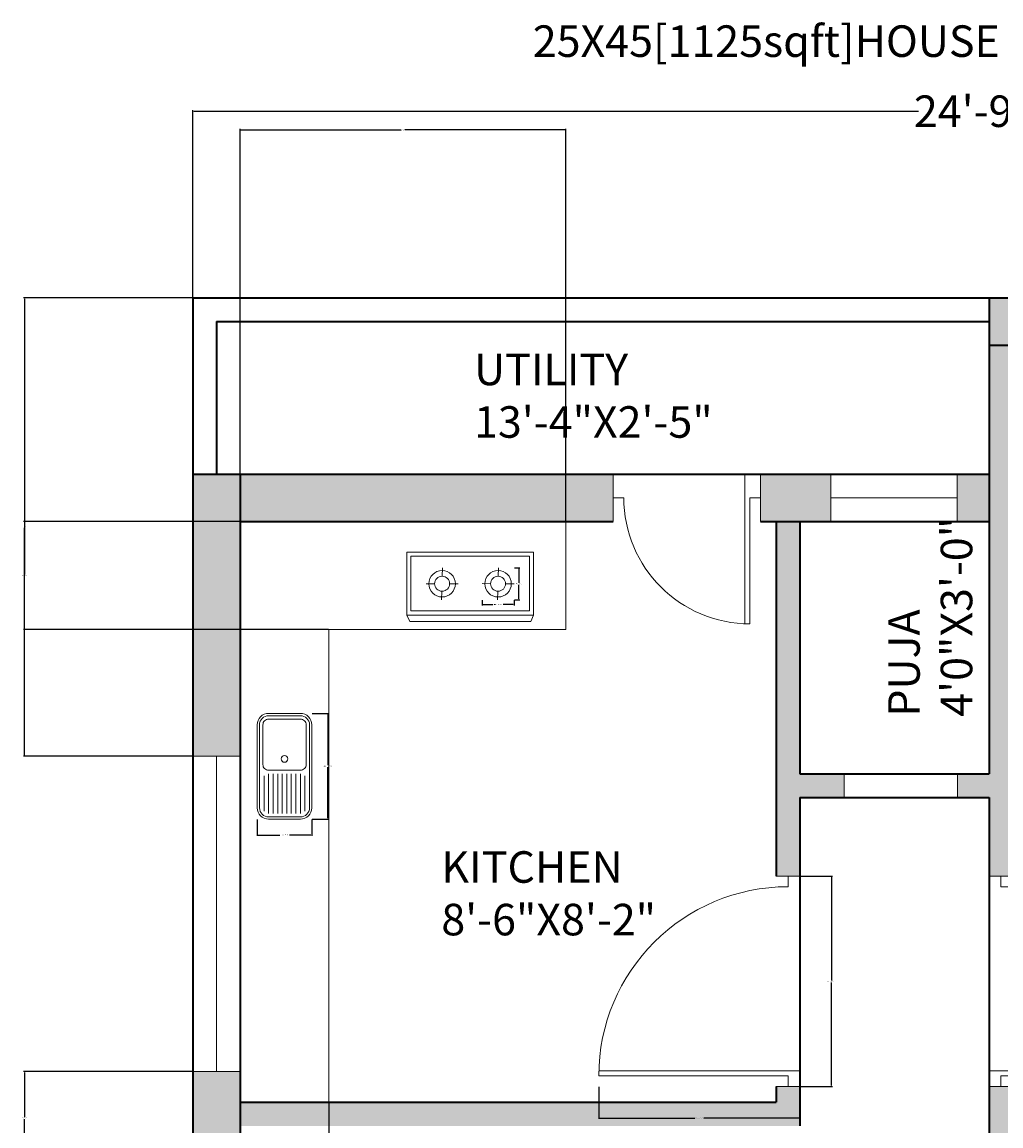
# Model space of a CAD drawing. Units: inches. Extents: x -13 to 349, y -556 to 61.
# Tile 5 of 6: x -13 to 174, y -149 to 61. Entities that reach past the tile are written whole.
import ezdxf

# ---------------------------------------------------------------- set-up
doc = ezdxf.new("R2010")
doc.units = ezdxf.units.IN
doc.header["$MEASUREMENT"] = 0
for name, color, linetype, lineweight in [('A-ANNO-DIMS', 2, 'Continuous', 18), ('A-ANNO-TEXT', 7, 'Continuous', 25), ('A-AREA-IDEN', 7, 'Continuous', 18), ('A-DOOR', 3, 'Continuous', 20), ('A-FLOR-CASE', 7, 'Continuous', 20), ('A-FLOR-OPEN', 1, 'Continuous', 13), ('A-GLAZ', 5, 'Continuous', 18), ('A-WALL', 7, 'Continuous', 35), ('A-WALL-PATT', 8, 'Continuous', 13), ('equipments', 7, 'Continuous', 18)]:
    doc.layers.add(name, color=color, linetype=linetype, lineweight=lineweight)
doc.styles.get("Standard").update_dxf_attribs({"font": 'arial.ttf'})
doc.dimstyles.get("Standard").update_dxf_attribs({"dimtxt": 0.18, "dimasz": 0.18, "dimexe": 0.18, "dimexo": 0.0625, "dimgap": 0.09, "dimtad": 0, "dimtih": 1, "dimtoh": 1, "dimdec": 0, "dimzin": 0, "dimdsep": 46, "dimlunit": 3, "dimtxsty": 'Standard', "dimcen": 0.09, "dimadec": 0, "dimazin": 0, "dimtfac": 1, "dimtdec": 0, "dimtofl": 0, "dimtmove": 0, "dimatfit": 3, "dimfxl": 1, "dimtolj": 1, "dimtzin": 0, "dimarcsym": 0})

# ---------------------------------------------------------------- blocks, each defined once
blk = doc.blocks.new('SINK_KITCHEN_SNGL')
for p, q in [((-39.5, -6), (-8.5, -6)), ((-36.5, -2), (36.5, -2)), ((-44.5, -38), (-44.5, -10)), ((-41.5, -10), (-6.5, -10)), ((-41.5, -14), (-6.5, -14)), ((-41.5, -18), (-6.5, -18)), ((44.5, -10), (44.5, -38)), ((-41.5, -22), (-6.5, -22)), ((-41.5, -26), (-6.5, -26)), ((-41.5, -30), (-6.5, -30)), ((-41.5, -34), (-6.5, -34)), ((-41.5, -38), (-6.5, -38)), ((-39.5, -42), (-8.5, -42)), ((36.5, -46), (-36.5, -46))]:
    blk.add_line(p, q)
at = {"flags": 128}
for points in [[(36.5, 0, -0.414214), (46.5, -10), (46.5, -38, -0.414214), (36.5, -48), (-36.5, -48, -0.414214), (-46.5, -38), (-46.5, -10, -0.414214), (-36.5, 0)], [(36.5, -5, -0.414214), (41.5, -10), (41.5, -38, -0.414214), (36.5, -43), (1.5, -43, -0.414214), (-3.5, -38), (-3.5, -10, -0.414214), (1.5, -5)]]:
    blk.add_lwpolyline(points, format="xyb", close=True, dxfattribs=at)
blk.add_circle((6.5, -24), 3)
for centre, start, end in [((-36.5, -10), 90, 180), ((36.5, -10), 0, 90), ((-36.5, -38), 180, 270), ((36.5, -38), 270, 0)]:
    blk.add_arc(centre, 8, start, end)
blk = doc.blocks.new('*D2')
at = {"layer": 'A-ANNO-DIMS', "color": 0, "lineweight": -2, "transparency": 16777216}
for p, q in [((19.76, 8.35), (19.76, 44)), ((19.94, 43.82), (157.81, 43.82)), ((316.58, 43.82), (178.7, 43.82)), ((316.76, 8.35), (316.76, 44))]:
    blk.add_line(p, q, dxfattribs=at)
at = {"layer": 'A-ANNO-DIMS', "color": 0, "transparency": 16777216}
for points in [[(19.94, 43.85), (19.94, 43.79), (19.76, 43.82)], [(316.58, 43.85), (316.58, 43.79), (316.76, 43.82)]]:
    blk.add_solid(points, dxfattribs=at)
at = {"layer": 'Defpoints', "color": 0, "transparency": 16777216}
for p in [(316.76, 43.82), (19.76, 8.29), (316.76, 8.29)]:
    blk.add_point(p, dxfattribs=at)
at = {"layer": 'A-ANNO-DIMS', "color": 0, "transparency": 16777216, "insert": (168.26, 43.82), "char_height": 6, "attachment_point": 5}
blk.add_mtext('\\A1;24\'-9"', dxfattribs=at)
blk = doc.blocks.new('DOOR-SWING-36IN')
for p, q in [((36, 40), (33.75, 40)), ((36, 38), (36, 40)), ((36, 40), (38.25, 40)), ((38.25, 3), (0, 3)), ((36, 2), (0, 2)), ((36, 0), (36, 2)), ((33.75, 0), (38.25, 0))]:
    blk.add_line(p, q)
blk.add_arc((36, 2), 36, 90, 180)
blk = doc.blocks.new('WIN-60IN-D9')
for p, q in [((0, 60), (0, 0)), ((9, 60), (0, 60)), ((4.5, 60), (4.5, 0)), ((9, 0), (9, 60)), ((0, 0), (9, 0))]:
    blk.add_line(p, q)
blk = doc.blocks.new('WIN-24IN-D9')
for p, q in [((0, 9), (24, 9)), ((0, 0), (0, 9)), ((24, 9), (24, 0)), ((0, 4.5), (24, 4.5)), ((24, 0), (0, 0))]:
    blk.add_line(p, q)
blk = doc.blocks.new('COOKTOP-BURNER')
for p, q in [((3.09, 4.48), (3.14, 6.09)), ((1.62, 3.06), (0, 3.06)), ((4.49, 3.04), (6.1, 3.03)), ((3.01, 1.61), (2.96, 0))]:
    blk.add_line(p, q)
for radius in [2.52, 1.43]:
    blk.add_circle((3.05, 3.05), radius)
blk = doc.blocks.new('*D14')
at = {"layer": 'A-ANNO-DIMS', "color": 0, "lineweight": -2, "transparency": 16777216}
for p, q in [((135.32, -101.71), (141.44, -101.71)), ((141.26, -101.89), (141.26, -121.53)), ((141.26, -141.53), (141.26, -121.9)), ((135.32, -141.71), (141.44, -141.71))]:
    blk.add_line(p, q, dxfattribs=at)
at = {"layer": 'A-ANNO-DIMS', "color": 0, "transparency": 16777216}
for points in [[(141.23, -101.89), (141.29, -101.89), (141.26, -101.71)], [(141.23, -141.53), (141.29, -141.53), (141.26, -141.71)]]:
    blk.add_solid(points, dxfattribs=at)
at = {"layer": 'Defpoints', "color": 0, "transparency": 16777216}
for p in [(135.26, -101.71), (141.26, -101.71), (135.26, -141.71)]:
    blk.add_point(p, dxfattribs=at)
at = {"layer": 'A-ANNO-DIMS', "color": 0, "transparency": 16777216, "insert": (141.26, -121.71), "char_height": 0.18, "attachment_point": 5}
blk.add_mtext('\\A1;D1 3\'-4" TYP.', dxfattribs=at)
blk = doc.blocks.new('*D15')
at = {"layer": 'A-ANNO-DIMS', "color": 0, "lineweight": -2, "transparency": 16777216}
for p, q in [((97.01, -141.78), (97.01, -147.89)), ((135.26, -141.78), (135.26, -147.89)), ((97.19, -147.71), (115.28, -147.71)), ((135.08, -147.71), (116.98, -147.71))]:
    blk.add_line(p, q, dxfattribs=at)
at = {"layer": 'A-ANNO-DIMS', "color": 0, "transparency": 16777216}
for points in [[(97.19, -147.68), (97.19, -147.74), (97.01, -147.71)], [(135.08, -147.68), (135.08, -147.74), (135.26, -147.71)]]:
    blk.add_solid(points, dxfattribs=at)
at = {"layer": 'Defpoints', "color": 0, "transparency": 16777216}
for p in [(97.01, -141.71), (135.26, -141.71), (135.26, -147.71)]:
    blk.add_point(p, dxfattribs=at)
at = {"layer": 'A-ANNO-DIMS', "color": 0, "transparency": 16777216, "insert": (116.13, -147.71), "char_height": 0.18, "attachment_point": 5}
blk.add_mtext('\\A1;3\'-2 1/2" TYP.', dxfattribs=at)
blk = doc.blocks.new('*D26')
at = {"layer": 'A-ANNO-DIMS', "color": 0, "lineweight": -2, "transparency": 16777216}
for p, q in [((42.48, -70.74), (45.61, -70.74)), ((45.43, -70.92), (45.43, -80.61)), ((45.43, -90.68), (45.43, -80.98)), ((42.48, -90.86), (45.61, -90.86))]:
    blk.add_line(p, q, dxfattribs=at)
at = {"layer": 'A-ANNO-DIMS', "color": 0, "transparency": 16777216}
for points in [[(45.4, -70.92), (45.46, -70.92), (45.43, -70.74)], [(45.4, -90.68), (45.46, -90.68), (45.43, -90.86)]]:
    blk.add_solid(points, dxfattribs=at)
at = {"layer": 'Defpoints', "color": 0, "transparency": 16777216}
for p in [(42.41, -70.74), (45.43, -70.74), (42.41, -90.86)]:
    blk.add_point(p, dxfattribs=at)
at = {"layer": 'A-ANNO-DIMS', "color": 0, "transparency": 16777216, "insert": (45.43, -80.8), "char_height": 0.18, "attachment_point": 5}
blk.add_mtext('\\A1;SINK 1\'-8" TYP.', dxfattribs=at)
blk = doc.blocks.new('*D27')
at = {"layer": 'A-ANNO-DIMS', "color": 0, "lineweight": -2, "transparency": 16777216}
for p, q in [((32.03, -90.92), (32.03, -94.05)), ((42.41, -90.92), (42.41, -94.05)), ((32.21, -93.87), (36.3, -93.87)), ((42.23, -93.87), (38.14, -93.87))]:
    blk.add_line(p, q, dxfattribs=at)
at = {"layer": 'A-ANNO-DIMS', "color": 0, "transparency": 16777216}
for points in [[(32.21, -93.84), (32.21, -93.9), (32.03, -93.87)], [(42.23, -93.84), (42.23, -93.9), (42.41, -93.87)]]:
    blk.add_solid(points, dxfattribs=at)
at = {"layer": 'Defpoints', "color": 0, "transparency": 16777216}
for p in [(32.03, -90.86), (42.41, -90.86), (42.41, -93.87)]:
    blk.add_point(p, dxfattribs=at)
at = {"layer": 'A-ANNO-DIMS', "color": 0, "transparency": 16777216, "insert": (37.22, -93.87), "char_height": 0.18, "attachment_point": 5}
blk.add_mtext('\\A1;0\'-10 1/2" TYP.', dxfattribs=at)
blk = doc.blocks.new('*D28')
at = {"layer": 'A-ANNO-DIMS', "color": 0, "lineweight": -2, "transparency": 16777216}
for p, q in [((74.79, -49.18), (74.79, -50.21)), ((74.97, -50.03), (76.85, -50.03)), ((80.7, -50.03), (78.82, -50.03)), ((80.88, -49.18), (80.88, -50.21))]:
    blk.add_line(p, q, dxfattribs=at)
at = {"layer": 'A-ANNO-DIMS', "color": 0, "transparency": 16777216}
for points in [[(74.97, -50), (74.97, -50.06), (74.79, -50.03)], [(80.7, -50), (80.7, -50.06), (80.88, -50.03)]]:
    blk.add_solid(points, dxfattribs=at)
at = {"layer": 'Defpoints', "color": 0, "transparency": 16777216}
for p in [(74.79, -49.12), (74.79, -50.03), (80.88, -49.12)]:
    blk.add_point(p, dxfattribs=at)
at = {"layer": 'A-ANNO-DIMS', "color": 0, "transparency": 16777216, "insert": (77.84, -50.03), "char_height": 0.18, "attachment_point": 5}
blk.add_mtext('\\A1;RING 0\'-6" TYP.', dxfattribs=at)
blk = doc.blocks.new('*D29')
at = {"layer": 'A-ANNO-DIMS', "color": 0, "lineweight": -2, "transparency": 16777216}
for p, q in [((80.94, -43.03), (81.98, -43.03)), ((81.8, -43.21), (81.8, -45.89)), ((81.8, -48.94), (81.8, -46.25)), ((80.94, -49.12), (81.98, -49.12))]:
    blk.add_line(p, q, dxfattribs=at)
at = {"layer": 'A-ANNO-DIMS', "color": 0, "transparency": 16777216}
for points in [[(81.77, -43.21), (81.83, -43.21), (81.8, -43.03)], [(81.77, -48.94), (81.83, -48.94), (81.8, -49.12)]]:
    blk.add_solid(points, dxfattribs=at)
at = {"layer": 'Defpoints', "color": 0, "transparency": 16777216}
for p in [(80.88, -43.03), (80.88, -49.12), (81.8, -49.12)]:
    blk.add_point(p, dxfattribs=at)
at = {"layer": 'A-ANNO-DIMS', "color": 0, "transparency": 16777216, "insert": (81.8, -46.07), "char_height": 0.18, "attachment_point": 5}
blk.add_mtext('\\A1;0\'-6" TYP.', dxfattribs=at)
blk = doc.blocks.new('*D38')
at = {"layer": 'A-ANNO-DIMS', "color": 0, "lineweight": -2, "transparency": 16777216}
for p, q in [((28.76, -144.78), (28.76, -555.89)), ((45.63, -144.78), (45.63, -555.89)), ((28.94, -555.71), (36.87, -555.71)), ((45.45, -555.71), (37.51, -555.71))]:
    blk.add_line(p, q, dxfattribs=at)
at = {"layer": 'A-ANNO-DIMS', "color": 0, "transparency": 16777216}
for points in [[(28.94, -555.68), (28.94, -555.74), (28.76, -555.71)], [(45.45, -555.68), (45.45, -555.74), (45.63, -555.71)]]:
    blk.add_solid(points, dxfattribs=at)
at = {"layer": 'Defpoints', "color": 0, "transparency": 16777216}
for p in [(28.76, -144.71), (45.63, -144.71), (45.63, -555.71)]:
    blk.add_point(p, dxfattribs=at)
at = {"layer": 'A-ANNO-DIMS', "color": 0, "transparency": 16777216, "insert": (37.19, -555.71), "char_height": 0.18, "attachment_point": 5}
blk.add_mtext('\\A1;1\'-5"', dxfattribs=at)
blk = doc.blocks.new('*D39')
at = {"layer": 'A-ANNO-DIMS', "color": 0, "lineweight": -2, "transparency": 16777216}
for p, q in [((28.69, -34.21), (-12.42, -34.21)), ((-12.24, -34.39), (-12.24, -44.31)), ((-12.24, -54.59), (-12.24, -44.68)), ((45.56, -54.77), (-12.42, -54.77))]:
    blk.add_line(p, q, dxfattribs=at)
at = {"layer": 'A-ANNO-DIMS', "color": 0, "transparency": 16777216}
for points in [[(-12.27, -34.39), (-12.21, -34.39), (-12.24, -34.21)], [(-12.27, -54.59), (-12.21, -54.59), (-12.24, -54.77)]]:
    blk.add_solid(points, dxfattribs=at)
at = {"layer": 'Defpoints', "color": 0, "transparency": 16777216}
for p in [(28.76, -34.21), (-12.24, -54.77), (45.63, -54.77)]:
    blk.add_point(p, dxfattribs=at)
at = {"layer": 'A-ANNO-DIMS', "color": 0, "transparency": 16777216, "insert": (-12.24, -44.49), "char_height": 0.18, "attachment_point": 5}
blk.add_mtext('\\A1;1\'-8 1/2"', dxfattribs=at)
blk = doc.blocks.new('*D40')
at = {"layer": 'A-ANNO-DIMS', "color": 0, "lineweight": -2, "transparency": 16777216}
for p, q in [((28.76, -34.15), (28.76, 40.47)), ((28.94, 40.29), (59.42, 40.29)), ((90.57, 40.29), (60.08, 40.29)), ((90.75, -34.15), (90.75, 40.47))]:
    blk.add_line(p, q, dxfattribs=at)
at = {"layer": 'A-ANNO-DIMS', "color": 0, "transparency": 16777216}
for points in [[(28.94, 40.32), (28.94, 40.26), (28.76, 40.29)], [(90.57, 40.32), (90.57, 40.26), (90.75, 40.29)]]:
    blk.add_solid(points, dxfattribs=at)
at = {"layer": 'Defpoints', "color": 0, "transparency": 16777216}
for p in [(90.75, 40.29), (28.76, -34.21), (90.75, -34.21)]:
    blk.add_point(p, dxfattribs=at)
at = {"layer": 'A-ANNO-DIMS', "color": 0, "transparency": 16777216, "insert": (59.75, 40.29), "char_height": 0.18, "attachment_point": 5}
blk.add_mtext('\\A1;5\'-2"', dxfattribs=at)
blk = doc.blocks.new('*D43')
at = {"layer": 'A-ANNO-DIMS', "color": 0, "lineweight": -2, "transparency": 16777216}
for p, q in [((19.69, 8.29), (-12.42, 8.29)), ((-12.24, 8.11), (-12.24, -35.11)), ((-12.24, -78.7), (-12.24, -35.48)), ((19.69, -78.88), (-12.42, -78.88))]:
    blk.add_line(p, q, dxfattribs=at)
at = {"layer": 'A-ANNO-DIMS', "color": 0, "transparency": 16777216}
for points in [[(-12.27, 8.11), (-12.21, 8.11), (-12.24, 8.29)], [(-12.27, -78.7), (-12.21, -78.7), (-12.24, -78.88)]]:
    blk.add_solid(points, dxfattribs=at)
at = {"layer": 'Defpoints', "color": 0, "transparency": 16777216}
for p in [(19.76, 8.29), (-12.24, -78.88), (19.76, -78.88)]:
    blk.add_point(p, dxfattribs=at)
at = {"layer": 'A-ANNO-DIMS', "color": 0, "transparency": 16777216, "insert": (-12.24, -35.3), "char_height": 0.18, "attachment_point": 5}
blk.add_mtext('\\A1;7\'-3"', dxfattribs=at)
blk = doc.blocks.new('*D44')
at = {"layer": 'A-ANNO-DIMS', "color": 0, "lineweight": -2, "transparency": 16777216}
for p, q in [((19.69, -138.88), (-12.42, -138.88)), ((-12.24, -139.06), (-12.24, -147.56)), ((-12.24, -156.44), (-12.24, -147.93)), ((19.69, -156.62), (-12.42, -156.62))]:
    blk.add_line(p, q, dxfattribs=at)
at = {"layer": 'A-ANNO-DIMS', "color": 0, "transparency": 16777216}
for points in [[(-12.27, -139.06), (-12.21, -139.06), (-12.24, -138.88)], [(-12.27, -156.44), (-12.21, -156.44), (-12.24, -156.62)]]:
    blk.add_solid(points, dxfattribs=at)
at = {"layer": 'Defpoints', "color": 0, "transparency": 16777216}
for p in [(19.76, -138.88), (-12.24, -156.62), (19.76, -156.62)]:
    blk.add_point(p, dxfattribs=at)
at = {"layer": 'A-ANNO-DIMS', "color": 0, "transparency": 16777216, "insert": (-12.24, -147.75), "char_height": 0.18, "attachment_point": 5}
blk.add_mtext('\\A1;1\'-5 1/2"', dxfattribs=at)

msp = doc.modelspace()

# ---------------------------------------------------------------- hatches: boundary and pattern name
at = {"layer": 'A-WALL-PATT'}
h = msp.add_hatch(color=256, dxfattribs=at)
h.dxf.hatch_style = 1
h.paths.add_polyline_path([(316.76, 8.29), (171.26, 8.29), (171.26, -0.71), (307.76, -0.71), (307.76, -52.19), (316.76, -52.19)])
h.paths.add_polyline_path([(175.76, -0.71), (171.26, -0.71), (171.26, -82.21), (165.24, -82.21), (165.24, -86.71), (171.26, -86.71), (171.26, -101.71), (173.51, -101.71), (175.76, -101.71)])
h.paths.add_polyline_path([(171.26, -25.21), (165.17, -25.21), (165.17, -34.21), (171.26, -34.21)])
h.paths.add_polyline_path([(141.17, -25.21), (127.76, -25.21), (127.76, -34.21), (141.17, -34.21)])
h.paths.add_polyline_path([(28.76, -25.21), (24.26, -25.21), (19.76, -25.21), (19.76, -78.88), (28.76, -78.88)])
h.paths.add_polyline_path([(99.76, -29.71), (99.76, -25.21), (28.76, -25.21), (28.76, -34.21), (99.76, -34.21)])
h.paths.add_polyline_path([(135.26, -86.71), (143.68, -86.71), (143.68, -82.21), (135.26, -82.21), (135.26, -34.21), (130.76, -34.21), (130.76, -101.71), (133.01, -101.71), (135.26, -101.71)])
h.paths.add_polyline_path([(135.26, -141.71), (130.76, -141.71), (130.76, -144.71), (28.76, -144.71), (28.76, -149.21), (135.26, -149.21)])
h.paths.add_polyline_path([(28.76, -138.88), (19.76, -138.88), (19.76, -156.62), (28.76, -156.62)])
h.paths.add_polyline_path([(28.76, -192.62), (19.76, -192.62), (19.76, -271.06), (28.76, -271.06)])
h.paths.add_polyline_path([(28.76, -307.06), (19.76, -307.06), (19.76, -385.56), (28.76, -385.56)])
h.paths.add_polyline_path([(28.76, -445.56), (19.76, -445.56), (19.76, -523.71), (28.76, -523.71)])
h.paths.add_polyline_path([(307.76, -431.71), (261.76, -431.71), (261.76, -353.71), (264.76, -353.71), (264.76, -349.21), (175.76, -349.21), (175.76, -248.21), (173.51, -248.21), (171.26, -248.21), (171.26, -317.21), (168.26, -317.21), (168.26, -321.71), (171.26, -321.71), (171.26, -353.71), (257.26, -353.71), (257.26, -431.71), (171.26, -431.71), (171.26, -436.21), (307.76, -436.21)])
h.paths.add_polyline_path([(316.76, -424.85), (307.76, -424.85), (307.76, -436.21), (316.76, -436.21)])
h.paths.add_polyline_path([(316.76, -305.84), (307.76, -305.84), (307.76, -400.85), (316.76, -400.85)])
h.paths.add_polyline_path([(307.76, -349.21), (292.76, -349.21), (292.76, -351.46), (292.76, -353.71), (307.76, -353.71)], flags=17)
h.paths.add_polyline_path([(271.19, -200.71), (267.26, -200.71), (267.26, -186.96), (262.76, -186.96), (262.76, -200.71), (175.76, -200.71), (175.76, -180.21), (173.51, -180.21), (171.26, -180.21), (171.26, -208.21), (175.76, -208.21), (175.76, -205.21), (271.19, -205.21)])
h.paths.add_polyline_path([(316.76, -112.19), (307.76, -112.19), (307.76, -245.84), (316.76, -245.84)])
h.paths.add_polyline_path([(271.33, -144.71), (175.76, -144.71), (175.76, -141.71), (171.26, -141.71), (171.26, -152.21), (175.76, -152.21), (175.76, -149.21), (262.76, -149.21), (262.76, -162.96), (267.26, -162.96), (267.26, -149.21), (271.33, -149.21)])
h.paths.add_polyline_path([(307.76, -200.71), (307.19, -200.71), (307.19, -205.21), (307.76, -205.21)])
h.paths.add_polyline_path([(307.76, -144.71), (307.33, -144.71), (307.33, -149.21), (307.76, -149.21)])

# ---------------------------------------------------------------- linework, layer by layer
at = {"layer": 'A-DOOR'}
for p, q in [((99.76, -29.71), (99.76, -25.21)), ((124.76, -25.21), (124.76, -53.71)), ((127.76, -34.21), (127.76, -25.21)), ((127.76, -25.21), (127.76, -25.21)), ((101.76, -29.71), (99.76, -29.71)), ((99.76, -29.71), (99.76, -34.21)), ((127.76, -29.71), (125.76, -29.71)), ((125.76, -29.71), (125.76, -53.71))]:
    msp.add_line(p, q, dxfattribs=at)
msp.add_arc((125.76, -29.71), 24, 180, 270, dxfattribs=at)
at = {"layer": 'A-FLOR-CASE'}
for p, q in [((90.75, -34.21), (90.75, -54.77)), ((90.75, -54.77), (45.63, -54.77)), ((45.63, -54.77), (45.63, -144.71))]:
    msp.add_line(p, q, dxfattribs=at)
at = {"layer": 'A-FLOR-OPEN'}
for p, q in [((143.68, -82.21), (143.68, -86.71)), ((165.24, -82.21), (143.68, -82.21)), ((165.24, -86.71), (165.24, -82.21)), ((143.68, -86.71), (165.24, -86.71))]:
    msp.add_line(p, q, dxfattribs=at)
at = {"layer": 'A-WALL'}
for p, q in [((19.76, 8.29), (19.76, -523.71)), ((19.76, 8.29), (316.76, 8.29)), ((171.26, 8.29), (171.26, -82.21)), ((24.26, 3.79), (171.26, 3.79)), ((24.26, 3.79), (24.26, -25.21)), ((171.26, -0.71), (307.76, -0.71)), ((19.76, -25.21), (171.26, -25.21)), ((28.76, -25.21), (28.76, -523.71)), ((28.76, -34.21), (99.76, -34.21)), ((127.76, -34.21), (171.26, -34.21)), ((130.76, -34.21), (130.76, -101.71)), ((135.26, -34.21), (135.26, -82.21)), ((135.26, -82.21), (171.26, -82.21)), ((135.26, -86.71), (171.26, -86.71)), ((135.26, -86.71), (135.26, -149.21)), ((171.26, -86.71), (171.26, -317.21)), ((130.76, -141.71), (130.76, -144.71)), ((28.76, -144.71), (130.76, -144.71))]:
    msp.add_line(p, q, dxfattribs=at)
at = {"layer": 'equipments'}
for p, q in [((60.48, -40.05), (60.48, -52.03)), ((60.48, -40.05), (84.61, -40.05)), ((61.28, -40.85), (61.28, -51.22)), ((61.28, -40.85), (83.8, -40.85)), ((83.8, -40.85), (83.8, -51.22)), ((84.61, -40.05), (84.61, -52.03)), ((60.48, -52.03), (84.61, -52.03)), ((60.48, -52.03), (61.04, -53.26)), ((61.28, -51.22), (83.8, -51.22)), ((84.61, -52.03), (84.05, -53.26)), ((61.04, -53.26), (84.05, -53.26))]:
    msp.add_line(p, q, dxfattribs=at)

# ---------------------------------------------------------------- block references
at = {"layer": 'A-DOOR'}
msp.add_blockref('DOOR-SWING-36IN', (97.01, -141.71), dxfattribs=at)
at = {"layer": 'A-DOOR', "extrusion": (0, 0, -1), "zscale": -1}
msp.add_blockref('DOOR-SWING-36IN', (-209.5, -141.71), dxfattribs=at)
at = {"layer": 'A-GLAZ'}
for name, p in [('WIN-24IN-D9', (141.17, -34.21)), ('WIN-60IN-D9', (19.76, -138.88))]:
    msp.add_blockref(name, p, dxfattribs=at)
at = {"layer": 'equipments'}
msp.add_blockref('COOKTOP-BURNER', (64.15, -49.12), dxfattribs=at)
at = {"layer": 'equipments', "rotation": 180}
msp.add_blockref('COOKTOP-BURNER', (80.89, -43.02), dxfattribs=at)
at = {"layer": 'equipments', "xscale": -0.2163424892709517, "yscale": 0.2163424892709517, "zscale": 0.2163424892709517, "rotation": 270}
msp.add_blockref('SINK_KITCHEN_SNGL', (42.41, -80.8), dxfattribs=at)
msp.add_blockref('SINK_KITCHEN_SNGL', (42.41, -80.8), dxfattribs=at)

# ---------------------------------------------------------------- texts
at = {"layer": 'A-ANNO-TEXT', "insert": (84.45, 60.15), "char_height": 6, "attachment_point": 1}
msp.add_mtext('25X45[1125sqft]HOUSE PLAN-NORTH FACE-FP1063', dxfattribs=at)
at = {"layer": 'A-AREA-IDEN', "char_height": 6, "attachment_point": 1}
for s, insert in [('UTILITY\\P13\'-4"X2\'-5"', (73.28, -2.3)), ('KITCHEN\\P8\'-6"X8\'-2"', (67.05, -96.96))]:
    msp.add_mtext(s, dxfattribs=dict(at, insert=insert))
at = {"layer": 'A-AREA-IDEN', "insert": (152.06, -71.37), "char_height": 6, "attachment_point": 1, "rotation": 90}
msp.add_mtext('PUJA\\P4\'0"X3\'-0"', dxfattribs=at)

# ---------------------------------------------------------------- dimensions: what is measured, and where the dimension line sits
at = {"layer": 'A-ANNO-DIMS'}
for base, p1, p2, override, picture, middle in [((316.76, 43.82), (19.76, 8.29), (316.76, 8.29), {"dimtxt": 6, "dimclrd": 0, "dimclre": 0, "dimclrt": 0}, '*D2', (168.26, 43.82)), ((90.75, 40.29), (28.76, -34.21), (90.75, -34.21), {"dimdec": 1, "dimlfac": 1, "dimrnd": 0, "dimzin": 1, "dimdsep": 46, "dimlunit": 4, "dimfrac": 2}, '*D40', (59.75, 40.29)), ((45.63, -555.71), (28.76, -144.71), (45.63, -144.71), {"dimdec": 1, "dimlfac": 1, "dimrnd": 0, "dimzin": 1, "dimdsep": 46, "dimlunit": 4, "dimfrac": 2}, '*D38', (37.19, -555.71))]:
    dim = msp.add_linear_dim(base=base, p1=p1, p2=p2, dimstyle='Standard', override=override, dxfattribs=at)
    dim.commit()
    dim.dimension.update_dxf_attribs({"geometry": picture, "text_midpoint": middle})
for base, p1, p2, picture, middle in [((-12.24, -78.88), (19.76, 8.29), (19.76, -78.88), '*D43', (-12.24, -35.3)), ((-12.24, -54.77), (28.76, -34.21), (45.63, -54.77), '*D39', (-12.24, -44.49)), ((-12.24, -156.62), (19.76, -138.88), (19.76, -156.62), '*D44', (-12.24, -147.75))]:
    dim = msp.add_linear_dim(base=base, p1=p1, p2=p2, angle=90, dimstyle='Standard', override={"dimdec": 1, "dimlfac": 1, "dimrnd": 0, "dimzin": 1, "dimdsep": 46, "dimlunit": 4, "dimfrac": 2}, dxfattribs=at)
    dim.commit()
    dim.dimension.update_dxf_attribs({"geometry": picture, "text_midpoint": middle})
for base, p1, p2, angle, text, picture, middle in [((81.8, -49.12), (80.88, -43.03), (80.88, -49.12), 270, '<> TYP.', '*D29', (81.8, -46.07)), ((74.79, -50.03), (80.88, -49.12), (74.79, -49.12), 180, 'RING <> TYP.', '*D28', (77.84, -50.03)), ((45.43, -70.74), (42.41, -90.86), (42.41, -70.74), 90, 'SINK <> TYP.', '*D26', (45.43, -80.8)), ((141.26, -101.71), (135.26, -141.71), (135.26, -101.71), 90, 'D1 <> TYP.', '*D14', (141.26, -121.71))]:
    dim = msp.add_linear_dim(base=base, p1=p1, p2=p2, angle=angle, text=text, dimstyle='Standard', override={"dimdec": 1, "dimlfac": 1, "dimrnd": 0, "dimzin": 1, "dimdsep": 46, "dimlunit": 4, "dimfrac": 2}, dxfattribs=at)
    dim.commit()
    dim.dimension.update_dxf_attribs({"geometry": picture, "text_midpoint": middle})
for base, p1, p2, picture, middle in [((42.41, -93.87), (32.03, -90.86), (42.41, -90.86), '*D27', (37.22, -93.87)), ((135.25577516, -147.71326771), (97.00577516, -141.71326771), (135.25577516, -141.71326771), '*D15', (116.13077516, -147.71326771))]:
    dim = msp.add_linear_dim(base=base, p1=p1, p2=p2, text='<> TYP.', dimstyle='Standard', override={"dimdec": 1, "dimlfac": 1, "dimrnd": 0, "dimzin": 1, "dimdsep": 46, "dimlunit": 4, "dimfrac": 2}, dxfattribs=at)
    dim.commit()
    dim.dimension.update_dxf_attribs({"geometry": picture, "text_midpoint": middle})

doc.saveas('drawing.dxf')
